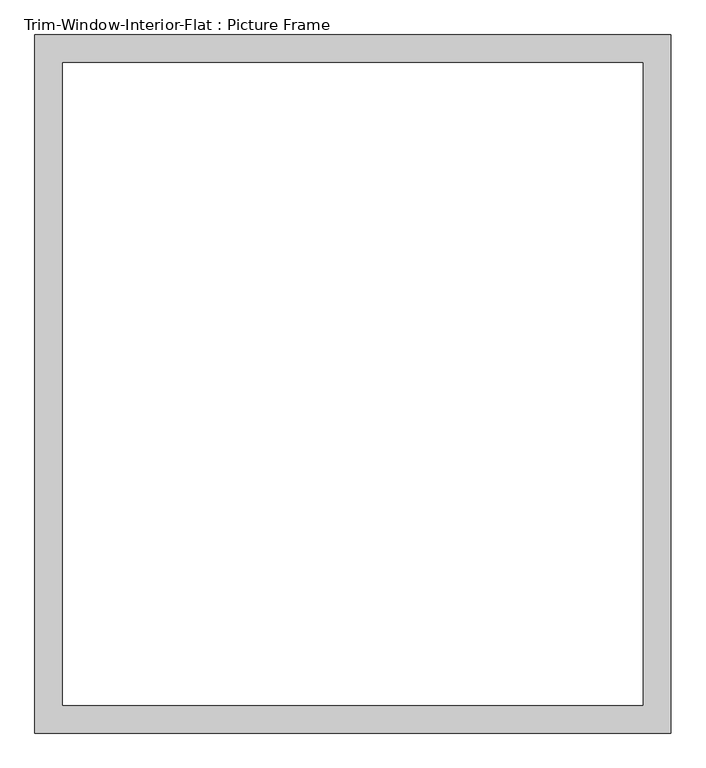
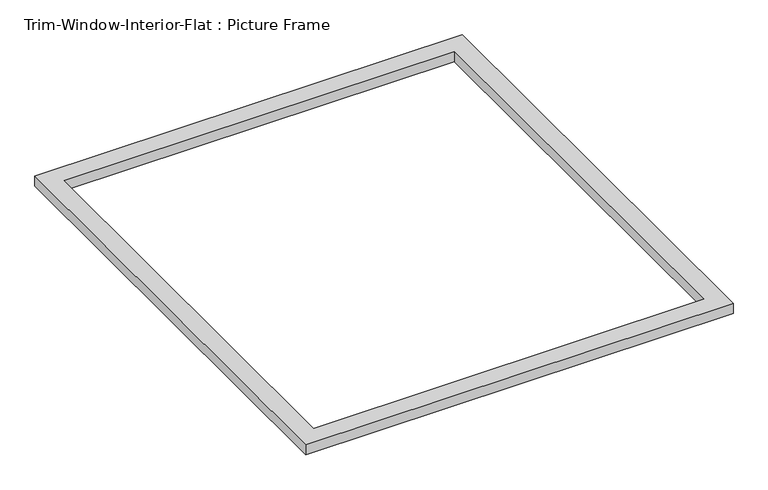
"""IFC4 building model written with IfcOpenShell, lengths in millimetres: proxy geometry, Trim-Window-Interior-Flat : Picture Frame."""

from ifc_helpers import new_model, si_unit, origin, origin_with_axes, place, context, project, spatial, polyline, outline, extrude, source, transform, mapped, element, save


def trim_window_interior_flat_picture_frame_a80dbcd9(model_context):
    return source(origin(), model_context, "Body", "SweptSolid", [
        extrude(outline(polyline([(654.05, 44.45), (654.05, -1390.65), (-654.05, -1390.65), (-654.05, 44.45), (654.05, 44.45)]), holes=[polyline([(596.9, -12.7), (-596.9, -12.7), (-596.9, -1333.5), (596.9, -1333.5), (596.9, -12.7)])]), origin_with_axes(), (0.0, 0.0, 1.0), 31.75),
    ])


if __name__ == "__main__":
    model = new_model("IFC4")
    model_context = context("Model", 3, world=origin())
    ifc_project = project(units=[si_unit("LENGTHUNIT", "METRE", prefix="MILLI")], contexts=[model_context])
    site = spatial("IfcSite", under=ifc_project)
    building = spatial("IfcBuilding", under=site)
    placement = place(None, origin())
    trim_window_interior_flat_picture_frame_shape = trim_window_interior_flat_picture_frame_a80dbcd9(model_context)
    element("IfcBuildingElementProxy", 1, Name="Trim-Window-Interior-Flat : Picture Frame", ObjectType="Trim-Window-Interior-Flat : Picture Frame", at=placement, inside=building, context=model_context, shape_type="MappedRepresentation", body=[
        mapped(trim_window_interior_flat_picture_frame_shape, transform((0.0, 0.0, 0.0), x_axis=(1.0, 0.0, 0.0), y_axis=(0.0, 1.0, 0.0), z_axis=(0.0, 0.0, 1.0))),
    ])
    save(model, "model.ifc")

# Revit data of these elements
# Type "Trim-Window-Interior-Flat : Picture Frame"
#   Trim Thickness_Picture Frame = 0' - 1 1/4"
#   Trim Width = 0' - 2 1/4"
#   Trim Thickness_with Sill = 0' - 0 3/4"
#   Sill Thickness = 0' - 1 1/4"
#   Opening Width [instance default] = 2' - 0"
#   Opening Height [instance default] = 3' - 0"
#   Default Elevation = 4' - 0"
#   Sill = no
#   Picture Frame = yes
#   Trim Material [instance default] = none
# Element 1 (IfcBuildingElementProxy, "Trim-Window-Interior-Flat : Picture Frame")
#   Opening Width = 4' - 0"
#   Opening Height = 4' - 5"
#   Trim Material = Wood - Stained
#   Materials on its faces: "Wood - Stained"
# Materials
#   "Wood - Stained": class "Wood", colour RGB 224 178 126, transparency 0, Cost = 0
